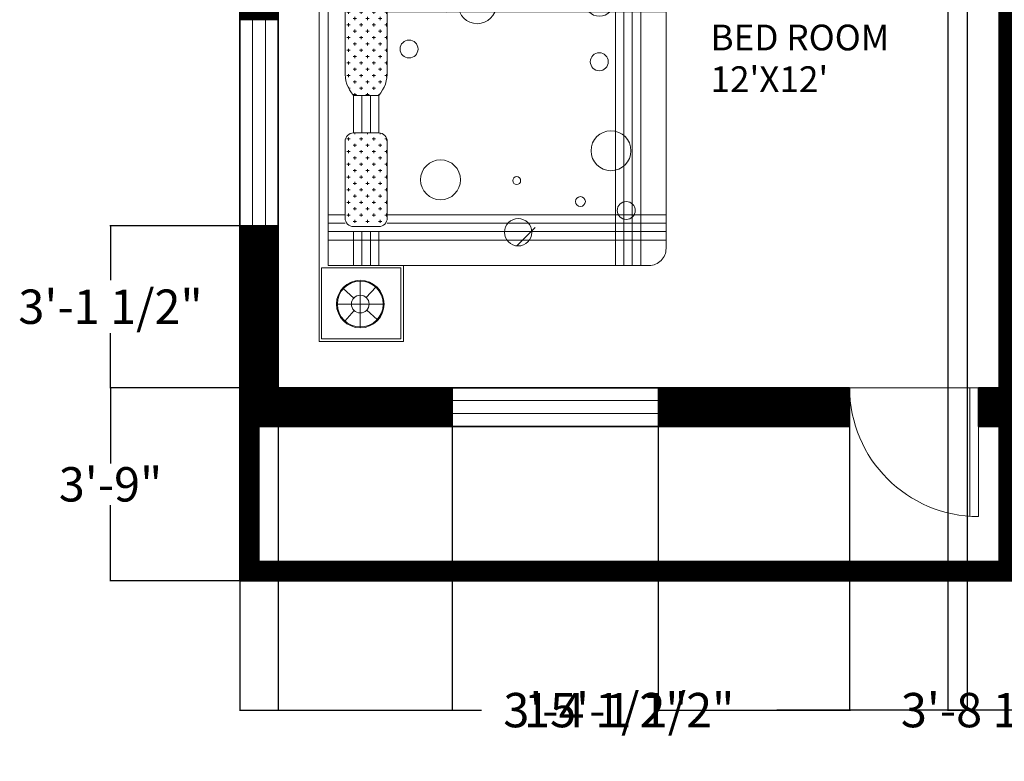
# Model space of a CAD drawing. Units: inches. Extents: x 108 to 771, y 58 to 590.
# Tile 1 of 8: x 111 to 341, y 58 to 231. Entities that reach past the tile are written whole.
import ezdxf

# ---------------------------------------------------------------- set-up
doc = ezdxf.new("R2010")
doc.units = ezdxf.units.IN
doc.header["$MEASUREMENT"] = 0
for name, color, linetype, lineweight in [('A-ANNO-DIMS', 2, 'Continuous', 13), ('A-AREA-IDEN', 7, 'Continuous', 18), ('A-DOOR', 3, 'Continuous', 18), ('A-GLAZ', 4, 'Continuous', 18), ('A-WALL', 7, 'Continuous', 35), ('A-WALL-PATT', 252, 'Continuous', 9), ('Furniture', 7, 'Continuous', 15)]:
    doc.layers.add(name, color=color, linetype=linetype, lineweight=lineweight)
doc.styles.get("Standard").update_dxf_attribs({"font": 'italic8.shx'})
doc.dimstyles.get("Standard").update_dxf_attribs({"dimtxt": 8, "dimasz": 0.18, "dimexe": 0.18, "dimexo": 0.0625, "dimgap": 0.09, "dimtad": 0, "dimtih": 1, "dimtoh": 1, "dimzin": 0, "dimdsep": 46, "dimlunit": 3, "dimtxsty": 'Standard', "dimcen": 0.09, "dimclrt": 6, "dimadec": 0, "dimazin": 0, "dimtfac": 1, "dimtofl": 0, "dimtmove": 0, "dimatfit": 3, "dimfxl": 1, "dimtolj": 1, "dimtzin": 0, "dimarcsym": 0})

# ---------------------------------------------------------------- blocks, each defined once
blk = doc.blocks.new('DOOR-SINGLE-30')
for p, q in [((28, 29.93), (28, 0)), ((30, 30), (30, 0)), ((30, 0), (0, 0))]:
    blk.add_line(p, q)
blk.add_arc((30, 0), 30, 90, 180)
blk = doc.blocks.new('WINDOW-48')
for p, q in [((0, 48), (0, 0)), ((9, 48), (0, 48)), ((3, 48), (3, 0)), ((6, 48), (6, 0)), ((9, 0), (9, 48)), ((0, 0), (9, 0))]:
    blk.add_line(p, q)
blk = doc.blocks.new('BED-WITH-NIGHTSTANDS')
h = blk.add_hatch()
h.set_pattern_fill('CROSS', color=256, scale=5.9055, angle=450, style=0)
h.set_pattern_definition([(90, (-724.7189, -618.2251), (1.476375, 1.476375), [0.7381875, -2.2145625]), (360, (-725.088, -617.856), (1.476375, -1.476375), [0.7381875, -2.2145625])])
h.paths.add_polyline_path([(13.93, 48.57), (8.02, 48.57, 0.414214), (6.06, 46.6), (6.06, 28.74, 0.414214), (8.02, 26.77), (13.93, 26.77, 0.414214), (15.9, 28.74), (15.9, 46.6, 0.414214)])
h.paths.add_polyline_path([(6.06, 62.99, 0.19223), (8.02, 57.33), (13.93, 57.33, 0.19223), (15.9, 62.99), (15.9, 78.74, 0.414214), (13.93, 80.71), (8.02, 80.71, 0.414214), (6.06, 78.74)])
for p, q in [((0, 0), (0, 106.3)), ((19.69, 106.3), (0, 106.3)), ((19.09, 105.71), (0.59, 105.71)), ((0.59, 105.71), (0.59, 89.17)), ((19.09, 105.71), (19.09, 89.17)), ((19.69, 106.3), (19.69, 88.58)), ((14.35, 103.55), (6.45, 100.09)), ((14.52, 103.48), (14.35, 103.55)), ((17.02, 97.76), (14.52, 103.48)), ((2.44, 101.15), (2.63, 101.34)), ((2.69, 100.86), (2.44, 101.15)), ((2.63, 101.34), (3.06, 101.2)), ((2.89, 101.55), (3.11, 101.7)), ((3.06, 101.2), (2.89, 101.55)), ((3.69, 101.46), (2.89, 100.92)), ((3.11, 101.7), (3.41, 101.48)), ((3.36, 101.88), (3.67, 101.95)), ((3.41, 101.48), (3.36, 101.88)), ((3.67, 101.95), (3.81, 101.64)), ((4.95, 101.56), (3.69, 101.46)), ((3.81, 101.64), (3.94, 101.98)), ((3.94, 101.98), (4.24, 102.02)), ((4.24, 102.02), (4.39, 101.64)), ((4.37, 102.03), (4.76, 102.08)), ((4.39, 101.64), (4.37, 102.03)), ((4.76, 102.08), (4.88, 101.72)), ((4.88, 101.72), (5.13, 102.07)), ((5.79, 101.48), (4.95, 101.56)), ((5.13, 102.07), (5.37, 102.03)), ((5.37, 102.03), (5.42, 101.66)), ((5.42, 101.66), (5.65, 101.97)), ((5.65, 101.97), (5.95, 101.95)), ((5.86, 101.55), (5.79, 101.48)), ((5.92, 101.48), (5.86, 101.55)), ((6.5, 101.45), (5.92, 101.48)), ((5.95, 101.95), (5.98, 101.59)), ((5.98, 101.59), (6.16, 101.92)), ((6.16, 101.92), (6.47, 101.91)), ((6.47, 101.91), (6.46, 101.54)), ((6.46, 101.54), (6.62, 101.9)), ((7.29, 101.35), (6.5, 101.45)), ((6.62, 101.9), (6.85, 101.89)), ((6.85, 101.89), (6.89, 101.51)), ((6.89, 101.51), (7.15, 101.84)), ((7.15, 101.84), (7.36, 101.82)), ((7.73, 101.29), (7.29, 101.35)), ((14.21, 102.94), (7.34, 99.94)), ((7.36, 101.82), (7.4, 101.48)), ((7.4, 101.48), (7.62, 101.8)), ((7.62, 101.8), (7.77, 101.81)), ((7.79, 101.48), (7.73, 101.29)), ((7.77, 101.81), (7.86, 101.7)), ((7.84, 101.37), (7.79, 101.48)), ((7.94, 101.33), (7.84, 101.37)), ((7.86, 101.7), (7.96, 101.49)), ((8.11, 101.22), (7.94, 101.33)), ((7.96, 101.49), (8.25, 101.43)), ((8.26, 101.14), (8.11, 101.22)), ((8.25, 101.43), (8.4, 101.32)), ((8.4, 100.95), (8.26, 101.14)), ((8.4, 101.32), (8.57, 101.02)), ((10.11, 100.6), (11.2, 101.08)), ((11.77, 101.33), (11.2, 101.08)), ((11.28, 100.91), (13.85, 102.03)), ((11.68, 99.99), (14.25, 101.12)), ((12.15, 101.56), (11.77, 101.33)), ((12.36, 101.86), (12.15, 101.56)), ((12.6, 102.1), (12.36, 101.86)), ((14.14, 102.78), (12.6, 102.1)), ((14.14, 102.78), (13.85, 102.03)), ((13.85, 102.03), (13.99, 102.03)), ((13.99, 102.03), (14.61, 102.64)), ((13.99, 102.03), (14.34, 101.23)), ((14.4, 102.82), (14.14, 102.78)), ((14.62, 102.78), (14.21, 102.94)), ((14.25, 101.12), (14.34, 101.23)), ((15, 100.83), (14.25, 101.12)), ((14.34, 101.23), (15.21, 101.26)), ((14.61, 102.64), (14.4, 102.82)), ((15.21, 101.26), (14.61, 102.64)), ((15.37, 101.06), (14.62, 102.78)), ((15.2, 100.99), (15, 100.83)), ((15.18, 100.71), (15.37, 101.06)), ((15.21, 101.26), (15.2, 100.99)), ((2.06, 100.15), (2.14, 100.41)), ((2.46, 100.04), (2.06, 100.15)), ((2.09, 99.7), (2.1, 99.92)), ((2.44, 99.53), (2.09, 99.7)), ((2.1, 99.92), (2.46, 100.04)), ((2.13, 99.38), (2.44, 99.53)), ((2.17, 99.14), (2.13, 99.38)), ((2.14, 100.41), (2.51, 100.41)), ((2.59, 99.17), (2.17, 99.14)), ((2.23, 100.67), (2.3, 100.88)), ((2.51, 100.41), (2.23, 100.67)), ((2.29, 98.95), (2.59, 99.17)), ((2.4, 98.76), (2.29, 98.95)), ((2.3, 100.88), (2.69, 100.86)), ((2.78, 98.76), (2.4, 98.76)), ((2.53, 98.47), (2.78, 98.76)), ((2.89, 100.92), (2.62, 100.19)), ((2.62, 100.19), (2.62, 99.39)), ((2.62, 99.39), (2.98, 98.72)), ((2.98, 98.72), (3.58, 98.25)), ((6.16, 98.57), (6.77, 98.66)), ((6.45, 100.09), (6.38, 99.93)), ((6.38, 99.93), (6.92, 98.7)), ((6.77, 98.66), (7.17, 98.75)), ((7.34, 99.94), (7.12, 99.5)), ((7.12, 99.5), (7.41, 98.83)), ((7.17, 98.75), (7.65, 98.91)), ((7.72, 98.74), (7.22, 98.53)), ((7.23, 99.41), (7.24, 99.69)), ((8.09, 99.45), (7.23, 99.41)), ((7.47, 98.85), (7.23, 99.41)), ((7.24, 99.69), (7.44, 99.85)), ((7.44, 99.85), (8.99, 100.52)), ((7.44, 99.85), (8.18, 99.56)), ((7.83, 98.04), (7.55, 98.67)), ((7.65, 98.91), (7.72, 98.74)), ((8.18, 99.56), (8.09, 99.45)), ((8.09, 99.45), (8.45, 98.65)), ((11.28, 100.91), (8.18, 99.56)), ((8.26, 97.68), (15.18, 100.71)), ((11.68, 99.99), (8.58, 98.64)), ((8.99, 100.52), (9.33, 100.53)), ((9.33, 100.53), (9.69, 100.49)), ((9.69, 100.49), (10.11, 100.6)), ((9.84, 98.58), (10.08, 98.82)), ((10.08, 98.82), (10.29, 99.11)), ((10.29, 99.11), (10.66, 99.34)), ((10.66, 99.34), (11.75, 99.82)), ((12.33, 100.07), (11.75, 99.82)), ((12.75, 100.19), (12.33, 100.07)), ((13.11, 100.14), (12.75, 100.19)), ((13.45, 100.15), (13.11, 100.14)), ((13.3, 99.4), (13.47, 99.48)), ((13.5, 98.95), (13.3, 99.4)), ((15, 100.83), (13.45, 100.15)), ((15.58, 99.65), (13.46, 98.72)), ((13.46, 98.72), (14.18, 97.06)), ((13.47, 99.48), (13.67, 99.02)), ((13.67, 99.02), (13.5, 98.95)), ((13.64, 99.55), (13.81, 99.63)), ((13.84, 99.1), (13.64, 99.55)), ((13.81, 99.63), (14.01, 99.17)), ((14.01, 99.17), (13.84, 99.1)), ((13.99, 99.7), (14.16, 99.78)), ((14.19, 99.25), (13.99, 99.7)), ((14.16, 99.78), (14.36, 99.32)), ((14.36, 99.32), (14.19, 99.25)), ((14.33, 99.85), (14.5, 99.93)), ((14.53, 99.4), (14.33, 99.85)), ((14.5, 99.93), (14.7, 99.47)), ((14.7, 99.47), (14.53, 99.4)), ((14.67, 100), (14.84, 100.08)), ((14.87, 99.55), (14.67, 100)), ((14.84, 100.08), (15.04, 99.62)), ((15.04, 99.62), (14.87, 99.55)), ((15.02, 100.16), (15.19, 100.23)), ((15.22, 99.7), (15.02, 100.16)), ((15.19, 100.23), (15.39, 99.77)), ((15.39, 99.77), (15.22, 99.7)), ((16.3, 97.99), (15.58, 99.65)), ((2.71, 98.26), (2.53, 98.47)), ((3.07, 98.46), (2.71, 98.26)), ((2.96, 98.08), (3.07, 98.46)), ((3.2, 97.92), (2.96, 98.08)), ((3.49, 98.1), (3.2, 97.92)), ((3.41, 97.75), (3.49, 98.1)), ((3.69, 97.67), (3.41, 97.75)), ((3.58, 98.25), (4.33, 98.05)), ((3.95, 97.97), (3.69, 97.67)), ((4.03, 97.59), (3.95, 97.97)), ((4.36, 97.56), (4.03, 97.59)), ((4.33, 98.05), (5.08, 98.31)), ((4.48, 97.99), (4.36, 97.56)), ((4.67, 97.64), (4.48, 97.99)), ((5, 97.75), (4.67, 97.64)), ((5.05, 98.16), (5, 97.75)), ((5.26, 97.85), (5.05, 98.16)), ((5.08, 98.31), (5.33, 98.48)), ((5.53, 98), (5.26, 97.85)), ((5.33, 98.48), (5.57, 98.34)), ((5.6, 98.18), (5.53, 98)), ((5.57, 98.34), (5.87, 98.48)), ((5.68, 98.18), (5.6, 98.18)), ((5.98, 98.32), (5.68, 98.18)), ((5.87, 98.48), (6.16, 98.57)), ((6.58, 98.42), (5.98, 98.32)), ((7.22, 98.53), (6.58, 98.42)), ((7.01, 98.5), (8.89, 94.2)), ((7.49, 98.64), (7.84, 97.84)), ((8.45, 98.65), (7.83, 98.04)), ((7.83, 98.04), (8.04, 97.86)), ((7.84, 97.84), (8.26, 97.68)), ((8.04, 97.86), (8.29, 97.9)), ((8.09, 97.13), (8.43, 97.28)), ((8.34, 96.55), (8.09, 97.13)), ((8.29, 97.9), (8.58, 98.64)), ((8.29, 97.9), (9.84, 98.58)), ((8.68, 96.7), (8.34, 96.55)), ((8.43, 97.28), (8.68, 96.7)), ((8.44, 96.33), (8.78, 96.48)), ((8.58, 98.64), (8.45, 98.65)), ((8.78, 96.48), (9.03, 95.9)), ((9.05, 94.14), (16.96, 97.59)), ((10.58, 98.29), (10.24, 98.14)), ((10.24, 98.14), (10.44, 97.68)), ((10.44, 97.68), (10.78, 97.83)), ((10.78, 97.83), (10.58, 98.29)), ((10.93, 97.48), (10.59, 97.33)), ((10.59, 97.33), (10.74, 96.99)), ((10.74, 96.99), (11.08, 97.14)), ((11.18, 96.91), (10.84, 96.76)), ((10.84, 96.76), (10.99, 96.42)), ((11.08, 97.14), (10.93, 97.48)), ((10.99, 96.42), (11.33, 96.57)), ((11.33, 96.57), (11.18, 96.91)), ((11.56, 97.76), (11.22, 97.61)), ((11.22, 97.61), (11.37, 97.27)), ((11.37, 97.27), (11.71, 97.42)), ((11.81, 97.19), (11.47, 97.04)), ((11.47, 97.04), (11.62, 96.69)), ((11.71, 97.42), (11.56, 97.76)), ((11.62, 96.69), (11.96, 96.84)), ((12.06, 96.61), (11.72, 96.46)), ((11.72, 96.46), (11.87, 96.12)), ((11.96, 96.84), (11.81, 97.19)), ((12.19, 98.03), (11.85, 97.88)), ((11.85, 97.88), (12, 97.54)), ((12, 97.54), (12.34, 97.69)), ((12.21, 96.27), (12.06, 96.61)), ((12.44, 97.46), (12.1, 97.31)), ((12.1, 97.31), (12.25, 96.97)), ((12.34, 97.69), (12.19, 98.03)), ((12.25, 96.97), (12.59, 97.12)), ((12.69, 96.89), (12.35, 96.74)), ((12.35, 96.74), (12.5, 96.39)), ((12.59, 97.12), (12.44, 97.46)), ((12.82, 98.31), (12.48, 98.16)), ((12.48, 98.16), (12.63, 97.82)), ((12.5, 96.39), (12.84, 96.55)), ((12.63, 97.82), (12.97, 97.97)), ((12.84, 96.55), (12.69, 96.89)), ((13.07, 97.74), (12.73, 97.59)), ((12.73, 97.59), (12.88, 97.24)), ((12.97, 97.97), (12.82, 98.31)), ((12.88, 97.24), (13.22, 97.39)), ((13.32, 97.16), (12.98, 97.01)), ((12.98, 97.01), (13.13, 96.67)), ((13.22, 97.39), (13.07, 97.74)), ((13.13, 96.67), (13.47, 96.82)), ((13.47, 96.82), (13.32, 97.16)), ((14.18, 97.06), (16.3, 97.99)), ((16.96, 97.59), (17.02, 97.76)), ((8.69, 95.75), (8.44, 96.33)), ((9.03, 95.9), (8.69, 95.75)), ((8.79, 95.52), (9.13, 95.67)), ((9.04, 94.95), (8.79, 95.52)), ((8.89, 94.2), (9.05, 94.14)), ((9.38, 95.1), (9.04, 94.95)), ((9.13, 95.67), (9.38, 95.1)), ((11.43, 96.34), (11.09, 96.19)), ((11.09, 96.19), (11.24, 95.84)), ((11.24, 95.84), (11.58, 95.99)), ((11.58, 95.99), (11.43, 96.34)), ((11.87, 96.12), (12.21, 96.27)), ((19.09, 89.17), (0.59, 89.17)), ((0.59, 89.17), (19.09, 89.17)), ((2.12, 17.72), (2.12, 88.58)), ((2.12, 88.58), (76.92, 88.58)), ((55.34, 82.68), (55.28, 82.62)), ((80.86, 84.65), (80.86, 21.65)), ((6.07, 78.98), (6.07, 62.76)), ((6.07, 46.84), (6.07, 28.51)), ((6.07, 44.57), (6.06, 44.56)), ((50.36, 26.51), (46.1, 22.26)), ((19.09, 17.13), (0.59, 17.13)), ((0.59, 0.59), (0.59, 17.13)), ((76.92, 17.72), (2.12, 17.72)), ((19.09, 0.59), (19.09, 17.13)), ((19.69, 0), (19.69, 17.72)), ((9.61, 8.71), (9.61, 14.05)), ((8.07, 10.1), (5.65, 12.3)), ((11, 10.24), (13.2, 12.67)), ((9.61, 8.71), (4.26, 8.71)), ((8.22, 7.18), (6.02, 4.75)), ((9.61, 8.71), (14.95, 8.71)), ((9.61, 8.71), (9.61, 3.36)), ((11.14, 7.32), (13.56, 5.12)), ((19.69, 0), (0, 0)), ((19.09, 0.59), (0.59, 0.59))]:
    blk.add_line(p, q)
for points in [[(8.02, 88.58), (8.02, 80.71)], [(9.99, 80.71), (9.99, 88.58), (8.02, 88.58)], [(13.93, 80.71), (13.93, 88.58), (11.96, 88.58)], [(11.96, 88.58), (11.96, 80.71)], [(2.12, 80.71), (80.86, 80.71), (80.86, 82.68), (2.12, 82.68)], [(15.9, 76.77), (80.86, 76.77), (80.86, 78.74), (15.9, 78.74)], [(8.02, 57.33), (8.02, 48.57)], [(9.99, 48.57), (9.99, 57.33)], [(11.96, 57.33), (11.96, 48.57)], [(13.93, 48.57), (13.93, 57.33)], [(2.12, 29.53), (6.06, 29.53)], [(6.06, 27.56), (2.12, 27.56)], [(15.9, 29.53), (80.86, 29.53), (80.86, 27.56), (15.9, 27.56)], [(2.12, 25.59), (80.86, 25.59), (80.86, 23.62), (2.12, 23.62)], [(8.02, 25.59), (8.02, 17.72), (9.99, 17.72), (9.99, 25.59)], [(11.96, 25.59), (11.96, 17.72), (13.93, 17.72), (13.93, 25.59)]]:
    blk.add_lwpolyline(points)
for points in [[(69.05, 88.58), (69.05, 17.72), (71.02, 17.72), (71.02, 88.58)], [(72.98, 88.58), (72.98, 17.72), (74.95, 17.72), (74.95, 88.58)]]:
    blk.add_lwpolyline(points, close=True)
for points in [[(15.9, 62.99), (15.9, 78.74, 0.414214), (13.93, 80.71), (8.02, 80.71, 0.414214), (6.06, 78.74), (6.06, 62.99, 0.19223), (8.02, 57.33), (13.93, 57.33, 0.19223)], [(15.9, 28.74), (15.9, 46.6, 0.414214), (13.93, 48.57), (8.02, 48.57, 0.414214), (6.06, 46.6), (6.06, 28.74, 0.414214), (8.02, 26.77), (13.93, 26.77, 0.414214)]]:
    blk.add_lwpolyline(points, format="xyb", close=True)
for centre, radius in [((36.86, 78.44), 4.41), ((65.32, 79.25), 3.48), ((29.81, 77.62), 0.925), ((20.97, 68.13), 2.09), ((65.3, 65.16), 2.09), ((68.02, 44.43), 4.65), ((28.31, 37.66), 4.65), ((46.05, 37.48), 0.925), ((60.91, 32.6), 1.14), ((71.58, 30.51), 2.09), ((46.4, 25.43), 3.19), ((9.61, 8.71), 5.54), ((9.61, 8.71), 5.34), ((9.61, 8.71), 2.07)]:
    blk.add_circle(centre, radius)
for centre, start, end in [((76.92, 84.65), 0, 90), ((76.92, 21.65), 270, 0)]:
    blk.add_arc(centre, 3.94, start, end)
blk = doc.blocks.new('*D28')
at = {"layer": 'A-ANNO-DIMS', "color": 0, "lineweight": -2, "transparency": 16777216}
for p, q in [((293.04, 253.99), (293.04, 248.02)), ((332.04, 253.99), (332.04, 248.02)), ((293.04, 248.2), (292.86, 248.2)), ((331.86, 248.2), (293.22, 248.2))]:
    blk.add_line(p, q, dxfattribs=at)
at = {"layer": 'A-ANNO-DIMS', "color": 0, "transparency": 16777216}
for points in [[(293.22, 248.23), (293.22, 248.17), (293.04, 248.2)], [(331.86, 248.23), (331.86, 248.17), (332.04, 248.2)]]:
    blk.add_solid(points, dxfattribs=at)
at = {"layer": 'Defpoints', "color": 0, "transparency": 16777216}
for p in [(293.04, 254.05), (332.04, 254.05), (293.04, 248.2)]:
    blk.add_point(p, dxfattribs=at)
at = {"layer": 'A-ANNO-DIMS', "color": 6, "transparency": 16777216, "insert": (200.58, 248.2), "char_height": 8, "attachment_point": 5}
blk.add_mtext('\\A1;BEDROOM DOOR 3\'-3" TYP.', dxfattribs=at)
blk = doc.blocks.new('*D46')
at = {"layer": 'A-ANNO-DIMS', "color": 0, "lineweight": -2, "transparency": 16777216}
for p, q in [((162.35, 99.99), (162.35, 69.77)), ((343.85, 99.99), (343.85, 69.77)), ((162.53, 69.95), (218.72, 69.95)), ((343.67, 69.95), (287.47, 69.95))]:
    blk.add_line(p, q, dxfattribs=at)
at = {"layer": 'A-ANNO-DIMS', "color": 0, "transparency": 16777216}
for points in [[(162.53, 69.98), (162.53, 69.92), (162.35, 69.95)], [(343.67, 69.98), (343.67, 69.92), (343.85, 69.95)]]:
    blk.add_solid(points, dxfattribs=at)
at = {"layer": 'Defpoints', "color": 0, "transparency": 16777216}
for p in [(162.35, 100.05), (343.85, 100.05), (343.85, 69.95)]:
    blk.add_point(p, dxfattribs=at)
at = {"layer": 'A-ANNO-DIMS', "color": 6, "transparency": 16777216, "insert": (253.1, 69.95), "char_height": 8, "attachment_point": 5}
blk.add_mtext('\\A1;15\'-1 1/2"', dxfattribs=at)
blk = doc.blocks.new('*D48')
at = {"layer": 'A-ANNO-DIMS', "color": 0, "lineweight": -2, "transparency": 16777216}
for p, q in [((171.28, 145.05), (132.07, 145.05)), ((132.25, 144.87), (132.25, 127.4)), ((132.25, 100.23), (132.25, 117.7)), ((162.28, 100.05), (132.07, 100.05))]:
    blk.add_line(p, q, dxfattribs=at)
at = {"layer": 'A-ANNO-DIMS', "color": 0, "transparency": 16777216}
for points in [[(132.22, 144.87), (132.28, 144.87), (132.25, 145.05)], [(132.22, 100.23), (132.28, 100.23), (132.25, 100.05)]]:
    blk.add_solid(points, dxfattribs=at)
at = {"layer": 'Defpoints', "color": 0, "transparency": 16777216}
for p in [(132.25, 145.05), (171.35, 145.05), (162.35, 100.05)]:
    blk.add_point(p, dxfattribs=at)
at = {"layer": 'A-ANNO-DIMS', "color": 6, "transparency": 16777216, "insert": (132.25, 122.55), "char_height": 8, "attachment_point": 5}
blk.add_mtext('\\A1;3\'-9"', dxfattribs=at)
blk = doc.blocks.new('*D58')
at = {"layer": 'A-ANNO-DIMS', "color": 0, "lineweight": -2, "transparency": 16777216}
for p, q in [((171.28, 182.8), (132.07, 182.8)), ((132.25, 182.62), (132.25, 170.11)), ((132.25, 145.23), (132.25, 157.74)), ((171.28, 145.05), (132.07, 145.05))]:
    blk.add_line(p, q, dxfattribs=at)
at = {"layer": 'A-ANNO-DIMS', "color": 0, "transparency": 16777216}
for points in [[(132.22, 182.62), (132.28, 182.62), (132.25, 182.8)], [(132.22, 145.23), (132.28, 145.23), (132.25, 145.05)]]:
    blk.add_solid(points, dxfattribs=at)
at = {"layer": 'Defpoints', "color": 0, "transparency": 16777216}
for p in [(132.25, 182.8), (171.35, 182.8), (171.35, 145.05)]:
    blk.add_point(p, dxfattribs=at)
at = {"layer": 'A-ANNO-DIMS', "color": 6, "transparency": 16777216, "insert": (132.25, 163.93), "char_height": 8, "attachment_point": 5}
blk.add_mtext('\\A1;3\'-1 1/2"', dxfattribs=at)
blk = doc.blocks.new('*D59')
at = {"layer": 'A-ANNO-DIMS', "color": 0, "lineweight": -2, "transparency": 16777216}
for p, q in [((327.35, 538.99), (327.35, 69.77)), ((331.85, 538.99), (331.85, 69.77)), ((327.53, 69.95), (331.67, 69.95)), ((331.85, 69.95), (332.03, 69.95))]:
    blk.add_line(p, q, dxfattribs=at)
at = {"layer": 'A-ANNO-DIMS', "color": 0, "transparency": 16777216}
for points in [[(327.53, 69.98), (327.53, 69.92), (327.35, 69.95)], [(331.67, 69.98), (331.67, 69.92), (331.85, 69.95)]]:
    blk.add_solid(points, dxfattribs=at)
at = {"layer": 'Defpoints', "color": 0, "transparency": 16777216}
for p in [(327.35, 539.05), (331.85, 539.05), (331.85, 69.95)]:
    blk.add_point(p, dxfattribs=at)
at = {"layer": 'A-ANNO-DIMS', "color": 6, "transparency": 16777216, "insert": (365.26, 69.95), "char_height": 8, "attachment_point": 5}
blk.add_mtext('\\A1;0\'-4 1/2"', dxfattribs=at)
blk = doc.blocks.new('*D60')
at = {"layer": 'A-ANNO-DIMS', "color": 0, "lineweight": -2, "transparency": 16777216}
for p, q in [((171.35, 145.12), (171.35, 578.33)), ((171.53, 578.15), (234.87, 578.15)), ((339.17, 578.15), (275.82, 578.15)), ((339.35, 145.12), (339.35, 578.33))]:
    blk.add_line(p, q, dxfattribs=at)
at = {"layer": 'A-ANNO-DIMS', "color": 0, "transparency": 16777216}
for points in [[(171.53, 578.18), (171.53, 578.12), (171.35, 578.15)], [(339.17, 578.18), (339.17, 578.12), (339.35, 578.15)]]:
    blk.add_solid(points, dxfattribs=at)
at = {"layer": 'Defpoints', "color": 0, "transparency": 16777216}
for p in [(339.35, 578.15), (171.35, 145.05), (339.35, 145.05)]:
    blk.add_point(p, dxfattribs=at)
at = {"layer": 'A-ANNO-DIMS', "color": 6, "transparency": 16777216, "insert": (255.35, 578.15), "char_height": 8, "attachment_point": 5}
blk.add_mtext('\\A1;14\'-0"', dxfattribs=at)
blk = doc.blocks.new('*D67')
at = {"layer": 'A-ANNO-DIMS', "color": 0, "lineweight": -2, "transparency": 16777216}
for p, q in [((171.35, 144.99), (171.35, 69.77)), ((211.84, 144.99), (211.84, 69.77)), ((171.53, 69.95), (211.66, 69.95)), ((211.84, 69.95), (212.02, 69.95))]:
    blk.add_line(p, q, dxfattribs=at)
at = {"layer": 'A-ANNO-DIMS', "color": 0, "transparency": 16777216}
for points in [[(171.53, 69.98), (171.53, 69.92), (171.35, 69.95)], [(211.66, 69.98), (211.66, 69.92), (211.84, 69.95)]]:
    blk.add_solid(points, dxfattribs=at)
at = {"layer": 'Defpoints', "color": 0, "transparency": 16777216}
for p in [(171.35, 145.05), (211.84, 145.05), (211.84, 69.95)]:
    blk.add_point(p, dxfattribs=at)
at = {"layer": 'A-ANNO-DIMS', "color": 6, "transparency": 16777216, "insert": (245.25, 69.95), "char_height": 8, "attachment_point": 5}
blk.add_mtext('\\A1;3\'-4 1/2"', dxfattribs=at)
blk = doc.blocks.new('*D68')
at = {"layer": 'A-ANNO-DIMS', "color": 0, "lineweight": -2, "transparency": 16777216}
for p, q in [((259.84, 135.99), (259.84, 69.77)), ((304.47, 135.99), (304.47, 69.77)), ((260.02, 69.95), (304.29, 69.95)), ((304.47, 69.95), (304.65, 69.95))]:
    blk.add_line(p, q, dxfattribs=at)
at = {"layer": 'A-ANNO-DIMS', "color": 0, "transparency": 16777216}
for points in [[(260.02, 69.98), (260.02, 69.92), (259.84, 69.95)], [(304.29, 69.98), (304.29, 69.92), (304.47, 69.95)]]:
    blk.add_solid(points, dxfattribs=at)
at = {"layer": 'Defpoints', "color": 0, "transparency": 16777216}
for p in [(259.84, 136.05), (304.47, 136.05), (304.47, 69.95)]:
    blk.add_point(p, dxfattribs=at)
at = {"layer": 'A-ANNO-DIMS', "color": 6, "transparency": 16777216, "insert": (337.88, 69.95), "char_height": 8, "attachment_point": 5}
blk.add_mtext('\\A1;3\'-8 1/2"', dxfattribs=at)

msp = doc.modelspace()

# ---------------------------------------------------------------- hatches: boundary and pattern name
at = {"layer": 'A-WALL-PATT'}
h = msp.add_hatch(dxfattribs=at)
h.set_pattern_fill('ANSI31', color=256)
h.paths.add_polyline_path([(171.345, 461.548), (162.345, 461.548), (162.345, 390.901), (171.345, 390.901), (171.345, 393.51), (171.345, 402.553), (233.142, 402.553), (233.142, 407.053), (171.345, 407.053)])
h.paths.add_polyline_path([(331.845, 438.553), (336.68, 438.554), (336.68, 443.053), (331.845, 443.053), (331.845, 539.053), (365.02, 539.053), (365.02, 548.053), (280.772, 548.053), (280.772, 539.053), (327.345, 539.053), (327.345, 407.053), (325.63, 407.053), (325.63, 402.553), (331.845, 402.553)])
h.paths.add_polyline_path([(286.63, 407.053), (263.142, 407.053), (263.142, 402.553), (267.345, 402.553), (267.345, 352.303), (171.345, 352.303), (171.345, 360.901), (162.345, 360.901), (162.345, 336.026), (171.345, 336.026), (171.345, 347.803), (267.345, 347.803), (267.345, 293.053), (263.142, 293.053), (263.142, 288.553), (293.037, 288.553), (293.037, 293.053), (271.845, 293.053), (271.845, 402.553), (286.63, 402.553)])
h.paths.add_polyline_path([(466.018, 443.053), (424.345, 443.053), (424.345, 539.053), (453.584, 539.053), (453.584, 548.053), (395.02, 548.053), (395.02, 539.053), (419.845, 539.053), (420.71, 443.053), (372.68, 443.053), (372.68, 438.557), (420.751, 438.561), (421.075, 402.553), (422.061, 293.053), (419.994, 293.053), (419.994, 288.553), (426.124, 288.553), (426.124, 293.053), (424.345, 293.053), (424.345, 402.553), (424.345, 438.553), (466.018, 438.553)])
h.paths.add_polyline_path([(512.345, 539.053), (583.918, 539.053), (583.918, 548.053), (483.584, 548.053), (483.584, 539.053), (507.845, 539.053), (507.845, 443.053), (502.018, 443.053), (502.018, 438.553), (507.845, 438.553), (507.845, 402.553), (515.658, 402.553), (515.658, 407.053), (512.345, 407.053)])
h.paths.add_polyline_path([(232.772, 548.053), (162.345, 548.053), (162.345, 509.548), (171.345, 509.548), (171.345, 539.053), (232.772, 539.053)])
h.paths.add_polyline_path([(233.142, 293.053), (171.345, 293.053), (171.345, 306.026), (162.345, 306.026), (162.345, 230.8), (171.345, 230.8), (171.345, 288.553), (233.142, 288.553)])
h.paths.add_polyline_path([(359.994, 293.053), (332.037, 293.053), (332.037, 288.553), (339.345, 288.553), (339.345, 145.053), (334.469, 145.053), (334.469, 136.053), (339.345, 136.053), (339.345, 104.553), (166.845, 104.553), (166.845, 136.053), (211.837, 136.053), (211.837, 145.053), (171.345, 145.053), (171.345, 182.8), (162.345, 182.8), (162.345, 100.053), (343.845, 100.053), (343.845, 136.053), (400.886, 136.053), (400.886, 145.053), (348.345, 145.053), (348.345, 288.553), (359.994, 288.553)])
h.paths.add_polyline_path([(500.345, 288.553), (503.755, 288.553), (503.755, 293.053), (486.124, 293.053), (486.124, 288.553), (491.345, 288.553), (491.345, 145.053), (448.886, 145.053), (448.886, 136.053), (495.845, 136.053), (495.845, 100.053), (677.345, 100.053), (677.345, 186.265), (668.345, 186.265), (668.345, 145.053), (627.637, 145.053), (627.637, 136.053), (672.845, 136.053), (672.845, 104.278), (500.345, 104.539), (500.345, 136.053), (504.239, 136.053), (504.239, 145.053), (500.345, 145.053)])
h.paths.add_polyline_path([(580.913, 293.053), (572.345, 293.053), (572.345, 347.803), (668.345, 347.803), (668.345, 330.831), (677.345, 330.831), (677.345, 366.853), (668.345, 366.853), (668.345, 352.303), (572.345, 352.303), (572.345, 402.553), (580.418, 402.553), (580.418, 407.053), (554.658, 407.053), (554.658, 402.553), (567.845, 402.553), (567.845, 293.053), (542.755, 293.053), (542.755, 288.553), (580.913, 288.553)])
h.paths.add_polyline_path([(677.345, 300.831), (668.345, 300.831), (668.345, 293.053), (610.913, 293.053), (610.913, 288.553), (668.345, 288.553), (668.345, 234.265), (677.345, 234.265)])
h.paths.add_polyline_path([(304.469, 145.053), (259.837, 145.053), (259.837, 136.053), (304.469, 136.053)], flags=17)
h.paths.add_polyline_path([(579.637, 145.053), (534.239, 145.053), (534.239, 136.053), (579.637, 136.053)], flags=17)
h.paths.add_polyline_path([(677.345, 450.416), (668.345, 450.416), (668.345, 407.053), (610.418, 407.053), (610.418, 402.553), (668.345, 402.553), (668.345, 396.853), (677.345, 396.853)])
h.paths.add_polyline_path([(677.345, 548.053), (631.918, 548.053), (631.918, 539.053), (668.345, 539.053), (668.345, 498.416), (677.345, 498.416)])
h = msp.add_hatch(dxfattribs=at)
h.set_pattern_fill('ANSI31', color=256)
h.paths.add_polyline_path([(365.02, 548.053), (280.772, 548.053), (280.772, 539.053), (327.345, 539.053), (327.345, 407.053), (325.63, 407.053), (325.63, 402.553), (331.845, 402.553), (331.845, 438.553), (336.68, 438.554), (336.68, 443.053), (331.845, 443.053), (331.845, 539.053), (365.02, 539.053)])
h.paths.add_polyline_path([(453.584, 548.053), (395.02, 548.053), (395.02, 539.053), (419.845, 539.053), (420.71, 443.053), (372.68, 443.053), (372.68, 438.557), (420.751, 438.561), (421.075, 402.553), (422.061, 293.053), (419.994, 293.053), (419.994, 288.553), (426.124, 288.553), (426.124, 293.053), (424.345, 293.053), (424.345, 402.553), (424.345, 438.553), (466.018, 438.553), (466.018, 443.053), (424.345, 443.053), (424.345, 539.053), (453.584, 539.053)])
h.paths.add_polyline_path([(232.772, 548.053), (162.345, 548.053), (162.345, 509.548), (171.345, 509.548), (171.345, 539.053), (232.772, 539.053)])
h.paths.add_polyline_path([(171.345, 461.548), (162.345, 461.548), (162.345, 390.901), (171.345, 390.901), (171.345, 393.51), (171.345, 402.553), (233.142, 402.553), (233.142, 407.053), (171.345, 407.053)])
h.paths.add_polyline_path([(286.63, 407.053), (263.142, 407.053), (263.142, 402.553), (267.345, 402.553), (267.345, 352.303), (171.345, 352.303), (171.345, 360.901), (162.345, 360.901), (162.345, 336.026), (171.345, 336.026), (171.345, 347.803), (267.345, 347.803), (267.345, 293.053), (263.142, 293.053), (263.142, 288.553), (293.037, 288.553), (293.037, 293.053), (271.845, 293.053), (271.845, 402.553), (286.63, 402.553)])
h.paths.add_polyline_path([(171.345, 306.026), (162.345, 306.026), (162.345, 230.8), (171.345, 230.8), (171.345, 288.553), (233.142, 288.553), (233.142, 293.053), (171.345, 293.053)])
h.paths.add_polyline_path([(348.345, 288.553), (359.994, 288.553), (359.994, 293.053), (332.037, 293.053), (332.037, 288.553), (339.345, 288.553), (339.345, 145.053), (334.469, 145.053), (334.469, 136.053), (339.345, 136.053), (339.345, 104.553), (166.845, 104.553), (166.845, 136.053), (211.837, 136.053), (211.837, 145.053), (171.345, 145.053), (171.345, 182.8), (162.345, 182.8), (162.345, 100.053), (343.845, 100.053), (343.845, 136.053), (400.886, 136.053), (400.886, 145.053), (348.345, 145.053)])
h.paths.add_polyline_path([(503.755, 293.053), (486.124, 293.053), (486.124, 288.553), (491.345, 288.553), (491.345, 145.053), (448.886, 145.053), (448.886, 136.053), (495.845, 136.053), (495.845, 100.053), (677.345, 100.053), (677.345, 186.265), (668.345, 186.265), (668.345, 145.053), (627.637, 145.053), (627.637, 136.053), (672.845, 136.053), (672.845, 104.278), (500.345, 104.539), (500.345, 136.053), (504.239, 136.053), (504.239, 145.053), (500.345, 145.053), (500.345, 288.553), (503.755, 288.553)])
h.paths.add_polyline_path([(580.913, 293.053), (572.345, 293.053), (572.345, 347.803), (668.345, 347.803), (668.345, 330.831), (677.345, 330.831), (677.345, 366.853), (668.345, 366.853), (668.345, 352.303), (572.345, 352.303), (572.345, 402.553), (580.418, 402.553), (580.418, 407.053), (554.658, 407.053), (554.658, 402.553), (567.845, 402.553), (567.845, 293.053), (542.755, 293.053), (542.755, 288.553), (580.913, 288.553)])
h.paths.add_polyline_path([(677.345, 300.831), (668.345, 300.831), (668.345, 293.053), (610.913, 293.053), (610.913, 288.553), (668.345, 288.553), (668.345, 234.265), (677.345, 234.265)])
h.paths.add_polyline_path([(579.637, 145.053), (534.239, 145.053), (534.239, 136.053), (579.637, 136.053)], flags=17)
h.paths.add_polyline_path([(304.469, 145.053), (259.837, 145.053), (259.837, 136.053), (304.469, 136.053)], flags=17)
h.paths.add_polyline_path([(583.918, 548.053), (483.584, 548.053), (483.584, 539.053), (507.845, 539.053), (507.845, 443.053), (502.018, 443.053), (502.018, 438.553), (507.845, 438.553), (507.845, 402.553), (515.658, 402.553), (515.658, 407.053), (512.345, 407.053), (512.345, 539.053), (583.918, 539.053)])
h.paths.add_polyline_path([(677.345, 548.053), (631.918, 548.053), (631.918, 539.053), (668.345, 539.053), (668.345, 498.416), (677.345, 498.416)])
h.paths.add_polyline_path([(677.345, 450.416), (668.345, 450.416), (668.345, 407.053), (610.418, 407.053), (610.418, 402.553), (668.345, 402.553), (668.345, 396.853), (677.345, 396.853)])

# ---------------------------------------------------------------- linework, layer by layer
at = {"layer": 'A-WALL'}
for p, q in [((162.345, 100.053), (162.345, 548.053)), ((171.345, 145.053), (171.345, 288.553)), ((339.345, 145.053), (339.345, 288.553)), ((304.469, 145.053), (171.345, 145.053)), ((304.469, 136.053), (304.469, 145.053)), ((339.345, 145.053), (334.469, 145.053)), ((334.469, 136.053), (334.469, 145.053)), ((166.845, 104.553), (166.845, 136.053)), ((304.469, 136.053), (166.845, 136.053)), ((339.345, 136.053), (334.469, 136.053)), ((339.345, 104.553), (339.345, 136.053)), ((339.345, 104.553), (166.845, 104.553)), ((343.845, 100.053), (162.345, 100.053))]:
    msp.add_line(p, q, dxfattribs=at)

# ---------------------------------------------------------------- block references
at = {"layer": 'A-DOOR', "extrusion": (0, 0, -1), "zscale": -1, "rotation": 180}
msp.add_blockref('DOOR-SINGLE-30', (-304.469, 145.053), dxfattribs=at)
at = {"layer": 'A-GLAZ'}
for p, rotation in [((171.346, 230.799), 180), ((211.838, 145.053), 269.9999999999995)]:
    msp.add_blockref('WINDOW-48', p, dxfattribs=dict(at, rotation=rotation))
at = {"layer": 'Furniture', "rotation": 359.999821755453}
msp.add_blockref('BED-WITH-NIGHTSTANDS', (180.838, 155.84), dxfattribs=at)

# ---------------------------------------------------------------- texts
at = {"layer": 'A-AREA-IDEN'}
for s, p in [('BED ROOM', (272.059, 223.653)), ("12'X12'", (272.059, 213.939))]:
    msp.add_text(s, height=6, dxfattribs=at).set_placement(p)

# ---------------------------------------------------------------- dimensions: what is measured, and where the dimension line sits
at = {"layer": 'A-ANNO-DIMS'}
for base, p1, p2, picture, middle in [((339.345, 578.153), (171.345, 145.053), (339.345, 145.053), '*D60', (255.345, 578.153)), ((331.845, 69.953), (327.345, 539.053), (331.845, 539.053), '*D59', (365.258, 69.953)), ((211.837, 69.953), (171.345, 145.053), (211.837, 145.053), '*D67', (245.25, 69.953)), ((304.469, 69.953), (259.837, 136.053), (304.469, 136.053), '*D68', (337.882, 69.953)), ((343.845, 69.953), (162.345, 100.053), (343.845, 100.053), '*D46', (253.095, 69.953))]:
    dim = msp.add_linear_dim(base=base, p1=p1, p2=p2, dimstyle='Standard', override={"dimdec": 1, "dimlfac": 1, "dimrnd": 0, "dimzin": 1, "dimdsep": 46, "dimlunit": 4, "dimfrac": 2}, dxfattribs=at)
    dim.commit()
    dim.dimension.update_dxf_attribs({"geometry": picture, "text_midpoint": middle})
dim = msp.add_linear_dim(base=(293.037, 248.203), p1=(332.037, 254.053), p2=(293.037, 254.053), angle=180, text='BEDROOM DOOR <> TYP.', dimstyle='Standard', override={"dimdec": 1, "dimlfac": 1, "dimrnd": 0, "dimzin": 1, "dimdsep": 46, "dimlunit": 4, "dimfrac": 2}, dxfattribs=at)
dim.commit()
dim.dimension.update_dxf_attribs({"geometry": '*D28', "text_midpoint": (200.576, 248.203)})
for base, p1, p2, picture, middle in [((132.245, 182.8), (171.345, 145.053), (171.345, 182.8), '*D58', (132.245, 163.926)), ((132.245, 145.053), (162.345, 100.053), (171.345, 145.053), '*D48', (132.245, 122.553))]:
    dim = msp.add_linear_dim(base=base, p1=p1, p2=p2, angle=90, dimstyle='Standard', override={"dimdec": 1, "dimlfac": 1, "dimrnd": 0, "dimzin": 1, "dimdsep": 46, "dimlunit": 4, "dimfrac": 2}, dxfattribs=at)
    dim.commit()
    dim.dimension.update_dxf_attribs({"geometry": picture, "text_midpoint": middle})

doc.saveas('drawing.dxf')
